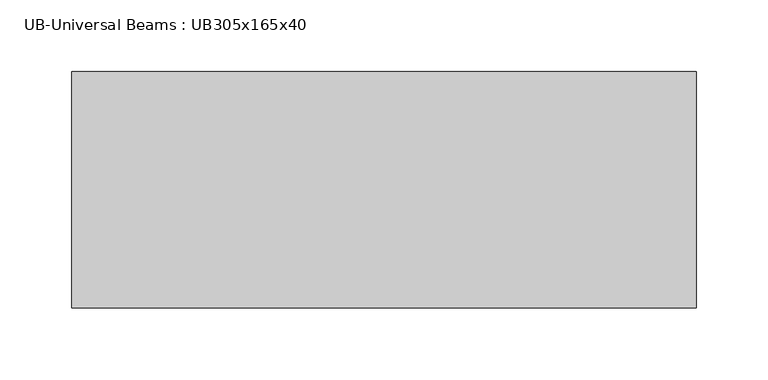
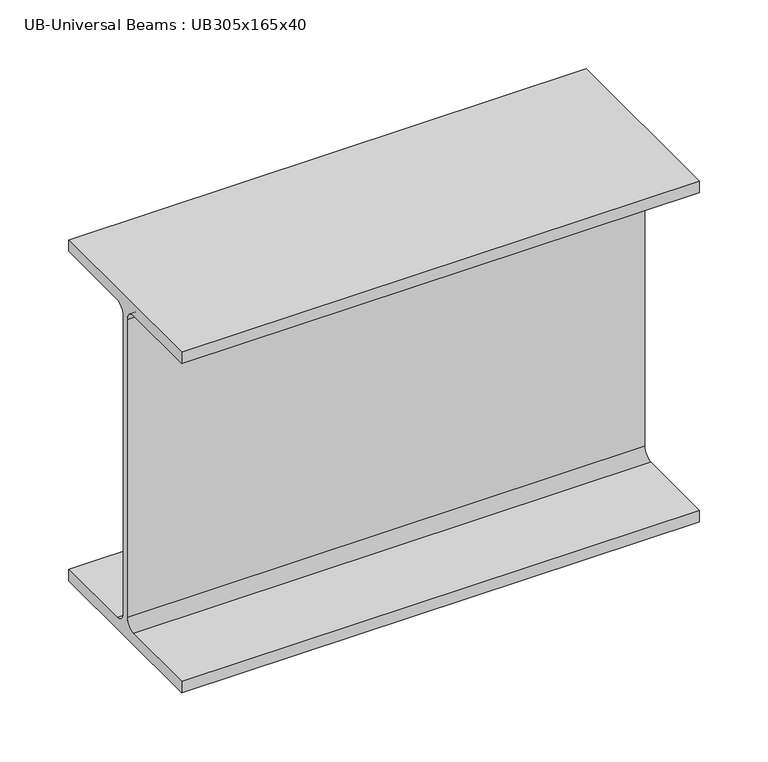
"""IFC4 building model written with IfcOpenShell, lengths in millimetres: beam geometry, UB-Universal Beams : UB305x165x40."""

from ifc_helpers import new_model, si_unit, point, frame, frame_2d, origin, place, context, project, spatial, polyline, circle_curve, trimmed, segment, composite_curve, outline, extrude, source, transform, mapped, element, save


def ub_universal_beams_ub305x165x40_05d28e63(model_context):
    return source(origin(), model_context, "Body", "SweptSolid", [
        extrude(outline(composite_curve([segment(polyline([(82.5, -141.5), (82.5, -151.7), (-82.5, -151.7), (-82.5, -141.5), (-11.9, -141.5)]), True, "CONTINUOUS"), segment(trimmed(circle_curve(frame_2d((-11.9, -132.6)), 8.9), [point((-11.9, -141.5))], [point((-3.0, -132.6))], True, "CARTESIAN"), True, "CONTINUOUS"), segment(polyline([(-3.0, -132.6), (-3.0, 132.6)]), True, "CONTINUOUS"), segment(trimmed(circle_curve(frame_2d((-11.9, 132.6)), 8.9), [point((-3.0, 132.6))], [point((-11.9, 141.5))], True, "CARTESIAN"), True, "CONTINUOUS"), segment(polyline([(-11.9, 141.5), (-82.5, 141.5), (-82.5, 151.7), (82.5, 151.7), (82.5, 141.5), (11.9, 141.5)]), True, "CONTINUOUS"), segment(trimmed(circle_curve(frame_2d((11.9, 132.6)), 8.9), [point((11.9, 141.5))], [point((3.0, 132.6))], True, "CARTESIAN"), True, "CONTINUOUS"), segment(polyline([(3.0, 132.6), (3.0, -132.6)]), True, "CONTINUOUS"), segment(trimmed(circle_curve(frame_2d((11.9, -132.6)), 8.9), [point((3.0, -132.6))], [point((11.9, -141.5))], True, "CARTESIAN"), True, "CONTINUOUS"), segment(polyline([(11.9, -141.5), (82.5, -141.5)]), True, "CONTINUOUS")], self_intersect=False)), frame((-230.7, 0.0, 0.0), z_axis=(1.0, 0.0, 0.0), x_axis=(0.0, 1.0, 0.0)), (0.0, 0.0, 1.0), 435.6),
    ])


if __name__ == "__main__":
    model = new_model("IFC4")
    model_context = context("Model", 3, world=origin())
    ifc_project = project(units=[si_unit("LENGTHUNIT", "METRE", prefix="MILLI")], contexts=[model_context])
    site = spatial("IfcSite", under=ifc_project)
    building = spatial("IfcBuilding", under=site)
    placement = place(None, origin())
    ub_universal_beams_ub305x165x40_shape = ub_universal_beams_ub305x165x40_05d28e63(model_context)
    element("IfcBeam", 1, ObjectType="UB-Universal Beams : UB305x165x40", at=placement, inside=building, context=model_context, shape_type="MappedRepresentation", body=[
        mapped(ub_universal_beams_ub305x165x40_shape, transform((0.0, 0.0, 0.0), x_axis=(1.0, 0.0, 0.0), y_axis=(0.0, 1.0, 0.0), z_axis=(0.0, 0.0, 1.0))),
    ])
    save(model, "model.ifc")

# Revit data of these elements
# Type "UB-Universal Beams : UB305x165x40"
#   Section Name Key = "UB305X165X40"
#   Width = 16.5 cm
#   Web Thickness = 0.6 cm
#   Web Fillet = 0.89 cm
#   Warping Constant = 164000.0 cm⁶
#   Torsional Moment of Inertia = 14.70 cm⁴
#   Section Area = 51.3 cm²
#   Plastic Modulus weak axis = 142.0 cm³
#   Plastic Modulus strong axis = 623.0 cm³
#   Nominal Weight = 40.2999 kgf/m
#   Moment of Inertia weak axis = 764.00 cm⁴
#   Moment of Inertia strong axis = 8503.00 cm⁴
#   Height = 30.34 cm
#   Flange Thickness = 1.02 cm
#   Elastic Modulus weak axis = 92.6 cm³
#   Elastic Modulus strong axis = 560.0 cm³
#   Centroid Vertical = 15.17 cm
#   Centroid Horizontal = 8.25 cm
#   Bolt Spacing = 9.0 cm
#   Length [instance default] = 1500 mm
#   Structural Material [instance default] = Metal - Steel 43-275
#   Type Comments = ""
#   Assembly Code = ""
# Element 1 (IfcBeam, "UB-Universal Beams : UB305x165x40")
#   Materials on its faces: "Metal - Steel 43-275"
# Materials
#   "Metal - Steel 43-275": class "Metal", colour RGB 247 247 247, transparency 0, Cost = 0
